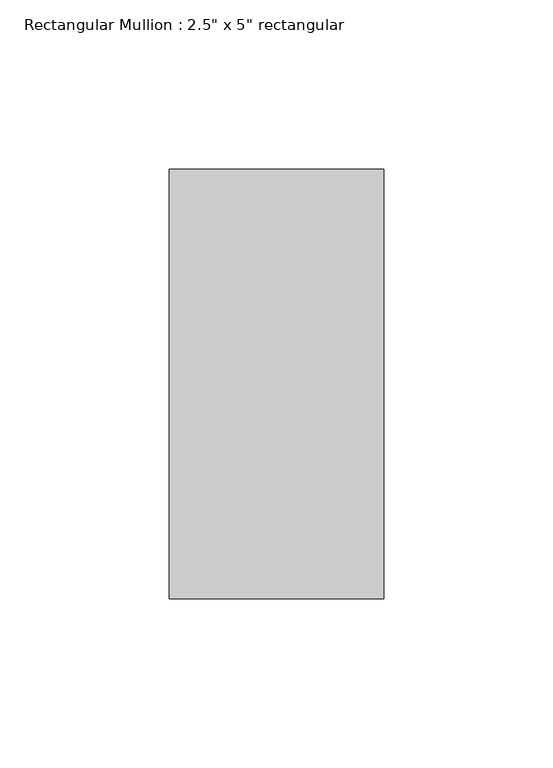
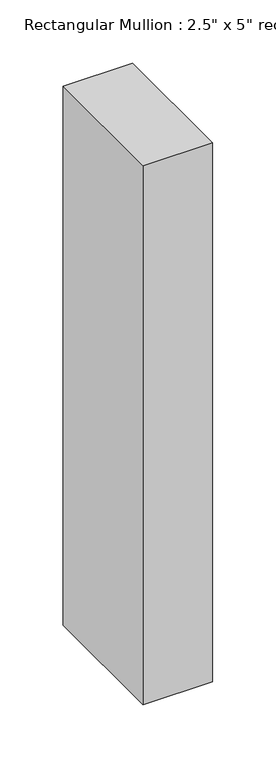
"""IFC4 building model written with IfcOpenShell, lengths in millimetres: member geometry."""

from ifc_helpers import new_model, si_unit, frame, origin, place, context, project, spatial, polyline, outline, extrude, source, transform, mapped, element, save


def member_8f80d2aa(model_context):
    return source(origin(), model_context, "Body", "SweptSolid", [
        extrude(outline(polyline([(0.0, 63.5), (0.0, -63.5), (-63.5, -63.5), (-63.5, 63.5), (0.0, 63.5)])), frame((0.0, 0.0, -520.7), z_axis=(0.0, 0.0, 1.0), x_axis=(1.0, 0.0, 0.0)), (0.0, 0.0, 1.0), 520.7),
    ])


if __name__ == "__main__":
    model = new_model("IFC4")
    model_context = context("Model", 3, world=origin())
    ifc_project = project(units=[si_unit("LENGTHUNIT", "METRE", prefix="MILLI")], contexts=[model_context])
    site = spatial("IfcSite", under=ifc_project)
    building = spatial("IfcBuilding", under=site)
    placement = place(None, origin())
    member_shape = member_8f80d2aa(model_context)
    element("IfcMember", 1, ObjectType="Rectangular Mullion : 2.5\" x 5\" rectangular", at=placement, inside=building, context=model_context, shape_type="MappedRepresentation", body=[
        mapped(member_shape, transform((0.0, 0.0, 0.0), x_axis=(1.0, 0.0, 0.0), y_axis=(0.0, 1.0, 0.0), z_axis=(0.0, 0.0, 1.0))),
    ])
    save(model, "model.ifc")

# Revit data of these elements
# Type "Rectangular Mullion : 2.5\" x 5\" rectangular"
#   built-in parameter 1007304 = 0.416667 (stored number, unit not read)
#   built-in parameter 1007301 = 0.104167 (stored number, unit not read)
#   built-in parameter 1007300 = 0.104167 (stored number, unit not read)
# Element 1 (IfcMember, "Rectangular Mullion : 2.5\" x 5\" rectangular")
#   Materials on its faces: "Aluminum"
# Materials
#   "Aluminum": class "Metal", colour RGB 247 247 247, transparency 0, Description = "Aluminum 6061", Cost = 0
